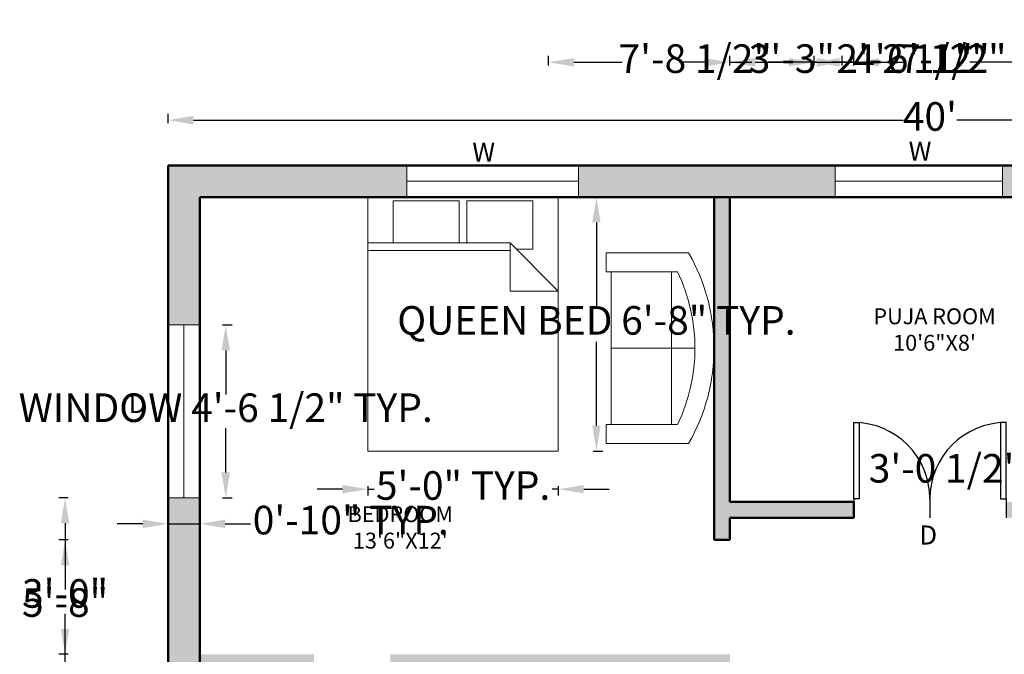
# Model space of a CAD drawing. Units: inches. Extents: x 2568 to 3190, y 746 to 1467.
# Tile 6 of 7: x 2588 to 2898, y 1267 to 1467. Entities that reach past the tile are written whole.
import ezdxf

# ---------------------------------------------------------------- set-up
doc = ezdxf.new("R2010")
doc.units = ezdxf.units.IN
for name, color, linetype, lineweight in [('A-ANNO-DIMS', 2, 'Continuous', 18), ('A-ANNO-TEXT', 7, 'Continuous', 18), ('A-AREA-IDEN', 7, 'Continuous', 25), ('A-DOOR', 3, 'Continuous', 25), ('A-FURN', 8, 'Continuous', 18), ('A-GLAZ', 4, 'Continuous', 20), ('A-WALL', 7, 'Continuous', 50), ('A-WALL-PATT', 252, 'Continuous', 13)]:
    doc.layers.add(name, color=color, linetype=linetype, lineweight=lineweight)
doc.styles.get("Standard").update_dxf_attribs({"font": 'arial.ttf'})
doc.dimstyles.new('ISO-25', dxfattribs={"dimtxt": 9, "dimasz": 8, "dimexe": 2, "dimexo": 1, "dimtad": 0, "dimtih": 1, "dimtoh": 1, "dimdec": 1, "dimlunit": 3, "dimtxsty": 'Standard', "dimcen": 2.5, "dimclrd": 1, "dimclre": 3, "dimclrt": 6, "dimadec": 0, "dimazin": 0, "dimtfac": 1, "dimtdec": 1, "dimtmove": 0, "dimatfit": 3, "dimfxl": 1, "dimfxlon": 1, "dimarcsym": 0})

# ---------------------------------------------------------------- blocks, each defined once
blk = doc.blocks.new('*U2')
for p, q in [((-24, 0), (-24, -6)), ((0, 0), (0, -6))]:
    blk.add_line(p, q)
blk.add_lwpolyline([(0, 0), (0, 24), (-1.75, 24), (-1.75, 0)], close=True)
blk.add_arc((0, 0), 24, 90, 180)
blk = doc.blocks.new('*U3')
for p, q in [((0, 0), (0, -6)), ((24, 0), (24, -6))]:
    blk.add_line(p, q)
blk.add_lwpolyline([(0, 0), (0, 24), (1.75, 24), (1.75, 0)], close=True)
blk.add_arc((0, 0), 24, 0, 90)
blk = doc.blocks.new('Bed - Queen')
for p, q in [((0, -80.00003), (0, 0)), ((0, 0), (59.99999, 0)), ((59.99999, 0), (59.99999, -80.00003)), ((7.99999, -1.2), (28.79998, -1.2)), ((7.99999, -14.4), (7.99999, -1.2)), ((28.79998, -1.2), (28.79998, -14.4)), ((31.19999, -1.2), (51.99999, -1.2)), ((31.19999, -14.4), (31.19999, -1.2)), ((51.99999, -1.2), (51.99999, -16.4)), ((0, -14.4), (44.8, -14.4)), ((59.99999, -29.6), (44.8, -14.4)), ((44.8, -14.4), (44.8, -29.6)), ((44.8, -16.8), (0, -16.8)), ((51.99999, -16.4), (46.79936, -16.4)), ((44.8, -29.6), (59.99999, -29.6)), ((59.99999, -80.00003), (0, -80.00003))]:
    blk.add_line(p, q)
blk = doc.blocks.new('*D13')
at = {"layer": 'A-ANNO-DIMS', "color": 0, "lineweight": -2, "transparency": 16777216}
for p, q in [((2634.52, 1434.58), (2634.52, 1437.58)), ((3114.52, 1434.58), (3114.52, 1437.58)), ((2642.52, 1435.58), (2866.08, 1435.58)), ((3106.52, 1435.58), (2882.97, 1435.58))]:
    blk.add_line(p, q, dxfattribs=at)
at = {"layer": 'A-ANNO-DIMS', "color": 0, "transparency": 16777216}
for points in [[(2642.52, 1436.91), (2642.52, 1434.24), (2634.52, 1435.58)], [(3106.52, 1436.91), (3106.52, 1434.24), (3114.52, 1435.58)]]:
    blk.add_solid(points, dxfattribs=at)
at = {"layer": 'Defpoints', "color": 0, "transparency": 16777216}
for p in [(2634.52, 1435.58), (2634.52, 1421.35), (3114.52, 1421.35)]:
    blk.add_point(p, dxfattribs=at)
at = {"layer": 'A-ANNO-DIMS', "color": 0, "transparency": 16777216, "insert": (2874.52, 1435.58), "char_height": 9, "attachment_point": 5}
blk.add_mtext("40'", dxfattribs=at)
blk = doc.blocks.new('Sofa - Roundback Loveseat 5 ft.')
for p, q in [((0, -32.44198), (0, -5.99998)), ((-24, -33.99998), (-24, -11.46958)), ((24.00004, -33.99998), (24.00004, -11.46958)), ((-23.9998, -13.38178), (23.99986, -13.38178)), ((-24, -32.44198), (24.00004, -32.44198))]:
    blk.add_line(p, q)
for points in [[(-24, -33.99998), (-30, -33.99998), (-30, -7.99998)], [(30.00004, -7.99998), (30.00004, -33.99998), (24.00004, -33.99998)]]:
    blk.add_lwpolyline(points)
for centre, radius, start, end in [((0, -60.24998), 60.24998, 60.13715, 119.8628), ((0, -61.38438), 55.38444, 64.32083, 115.6792)]:
    blk.add_arc(centre, radius, start, end)
blk = doc.blocks.new('WIN-BED-UPPER-54.46')
for p, q in [((5, 54.46), (-5, 54.46)), ((0, 54.46), (0, 0)), ((5, 0), (-5, 0))]:
    blk.add_line(p, q)
blk = doc.blocks.new('*D21')
at = {"layer": 'A-ANNO-DIMS', "color": 3, "lineweight": -2, "transparency": 16777216}
for p, q in [((2768.47, 1411.35), (2771.47, 1411.35)), ((2768.47, 1331.35), (2771.47, 1331.35))]:
    blk.add_line(p, q, dxfattribs=at)
at = {"layer": 'A-ANNO-DIMS', "color": 1, "lineweight": -2, "transparency": 16777216}
for p, q in [((2769.47, 1403.35), (2769.47, 1376.9)), ((2769.47, 1339.35), (2769.47, 1365.79))]:
    blk.add_line(p, q, dxfattribs=at)
at = {"layer": 'A-ANNO-DIMS', "color": 1, "transparency": 16777216}
for points in [[(2768.14, 1403.35), (2770.8, 1403.35), (2769.47, 1411.35)], [(2768.14, 1339.35), (2770.8, 1339.35), (2769.47, 1331.35)]]:
    blk.add_solid(points, dxfattribs=at)
at = {"layer": 'Defpoints', "color": 0, "transparency": 16777216}
for p in [(2757.47, 1411.35), (2769.47, 1411.35), (2757.47, 1331.35)]:
    blk.add_point(p, dxfattribs=at)
at = {"layer": 'A-ANNO-DIMS', "color": 6, "transparency": 16777216, "insert": (2769.47, 1371.35), "char_height": 9, "attachment_point": 5}
blk.add_mtext('QUEEN BED 6\'-8" TYP.', dxfattribs=at)
blk = doc.blocks.new('*D22')
at = {"layer": 'A-ANNO-DIMS', "color": 1, "lineweight": -2, "transparency": 16777216}
for p, q in [((2689.47, 1319.35), (2681.47, 1319.35)), ((2697.47, 1319.35), (2699.42, 1319.35)), ((2757.47, 1319.35), (2755.53, 1319.35)), ((2765.47, 1319.35), (2773.47, 1319.35))]:
    blk.add_line(p, q, dxfattribs=at)
at = {"layer": 'A-ANNO-DIMS', "color": 3, "lineweight": -2, "transparency": 16777216}
for p, q in [((2697.47, 1320.35), (2697.47, 1317.35)), ((2757.47, 1320.35), (2757.47, 1317.35))]:
    blk.add_line(p, q, dxfattribs=at)
at = {"layer": 'A-ANNO-DIMS', "color": 1, "transparency": 16777216}
for points in [[(2689.47, 1320.68), (2689.47, 1318.02), (2697.47, 1319.35)], [(2765.47, 1320.68), (2765.47, 1318.02), (2757.47, 1319.35)]]:
    blk.add_solid(points, dxfattribs=at)
at = {"layer": 'Defpoints', "color": 0, "transparency": 16777216}
for p in [(2697.47, 1331.35), (2757.47, 1331.35), (2757.47, 1319.35)]:
    blk.add_point(p, dxfattribs=at)
at = {"layer": 'A-ANNO-DIMS', "color": 6, "transparency": 16777216, "insert": (2727.47, 1319.35), "char_height": 9, "attachment_point": 5}
blk.add_mtext('5\'-0" TYP.', dxfattribs=at)
blk = doc.blocks.new('*D24')
at = {"layer": 'A-ANNO-DIMS', "color": 1, "lineweight": -2, "transparency": 16777216}
for p, q in [((2939.86, 1324.76), (2931.86, 1324.76)), ((2968.52, 1324.76), (2947.86, 1324.76))]:
    blk.add_line(p, q, dxfattribs=at)
at = {"layer": 'A-ANNO-DIMS', "color": 3, "lineweight": -2, "transparency": 16777216}
for p, q in [((2939.86, 1325.76), (2939.86, 1322.76)), ((2976.52, 1325.76), (2976.52, 1322.76))]:
    blk.add_line(p, q, dxfattribs=at)
at = {"layer": 'A-ANNO-DIMS', "color": 1, "transparency": 16777216}
for points in [[(2947.86, 1326.09), (2947.86, 1323.43), (2939.86, 1324.76)], [(2968.52, 1326.09), (2968.52, 1323.43), (2976.52, 1324.76)]]:
    blk.add_solid(points, dxfattribs=at)
at = {"layer": 'Defpoints', "color": 0, "transparency": 16777216}
for p in [(2939.86, 1333.76), (2976.52, 1333.76), (2939.86, 1324.76)]:
    blk.add_point(p, dxfattribs=at)
at = {"layer": 'A-ANNO-DIMS', "color": 6, "transparency": 16777216, "insert": (2893.32, 1324.76), "char_height": 9, "attachment_point": 5}
blk.add_mtext('3\'-0 1/2" TYP.', dxfattribs=at)
blk = doc.blocks.new('*D29')
at = {"layer": 'A-ANNO-DIMS', "color": 3, "lineweight": -2, "transparency": 16777216}
for p, q in [((2651.69, 1371.08), (2654.69, 1371.08)), ((2651.69, 1316.62), (2654.69, 1316.62))]:
    blk.add_line(p, q, dxfattribs=at)
at = {"layer": 'A-ANNO-DIMS', "color": 1, "lineweight": -2, "transparency": 16777216}
for p, q in [((2652.69, 1363.08), (2652.69, 1349.13)), ((2652.69, 1324.62), (2652.69, 1338.56))]:
    blk.add_line(p, q, dxfattribs=at)
at = {"layer": 'A-ANNO-DIMS', "color": 1, "transparency": 16777216}
for points in [[(2651.36, 1363.08), (2654.02, 1363.08), (2652.69, 1371.08)], [(2651.36, 1324.62), (2654.02, 1324.62), (2652.69, 1316.62)]]:
    blk.add_solid(points, dxfattribs=at)
at = {"layer": 'Defpoints', "color": 0, "transparency": 16777216}
for p in [(2644.52, 1371.08), (2652.69, 1371.08), (2644.52, 1316.62)]:
    blk.add_point(p, dxfattribs=at)
at = {"layer": 'A-ANNO-DIMS', "color": 6, "transparency": 16777216, "insert": (2652.69, 1343.85), "char_height": 9, "attachment_point": 5}
blk.add_mtext('WINDOW 4\'-6 1/2" TYP.', dxfattribs=at)
blk = doc.blocks.new('*D30')
at = {"layer": 'A-ANNO-DIMS', "color": 3, "lineweight": -2, "transparency": 16777216}
for p, q in [((2634.52, 1309.45), (2634.52, 1306.45)), ((2644.52, 1309.45), (2644.52, 1306.45))]:
    blk.add_line(p, q, dxfattribs=at)
at = {"layer": 'A-ANNO-DIMS', "color": 1, "lineweight": -2, "transparency": 16777216}
for p, q in [((2626.52, 1308.45), (2618.52, 1308.45)), ((2634.52, 1308.45), (2644.52, 1308.45)), ((2652.52, 1308.45), (2660.52, 1308.45))]:
    blk.add_line(p, q, dxfattribs=at)
at = {"layer": 'A-ANNO-DIMS', "color": 1, "transparency": 16777216}
for points in [[(2626.52, 1309.78), (2626.52, 1307.11), (2634.52, 1308.45)], [(2652.52, 1309.78), (2652.52, 1307.11), (2644.52, 1308.45)]]:
    blk.add_solid(points, dxfattribs=at)
at = {"layer": 'Defpoints', "color": 0, "transparency": 16777216}
for p in [(2634.52, 1316.62), (2644.52, 1316.62), (2644.52, 1308.45)]:
    blk.add_point(p, dxfattribs=at)
at = {"layer": 'A-ANNO-DIMS', "color": 6, "transparency": 16777216, "insert": (2692.07, 1308.45), "char_height": 9, "attachment_point": 5}
blk.add_mtext('0\'-10" TYP.', dxfattribs=at)
blk = doc.blocks.new('*D31')
at = {"layer": 'A-ANNO-DIMS', "color": 1, "lineweight": -2, "transparency": 16777216}
for p, q in [((2648.47, 1248.37), (2648.47, 1256.37)), ((2648.47, 1256.37), (2656.47, 1256.37)), ((2648.47, 1230.08), (2648.47, 1240.37))]:
    blk.add_line(p, q, dxfattribs=at)
at = {"layer": 'A-ANNO-DIMS', "color": 3, "lineweight": -2, "transparency": 16777216}
for p, q in [((2647.47, 1248.37), (2650.47, 1248.37)), ((2647.47, 1222.08), (2650.47, 1222.08))]:
    blk.add_line(p, q, dxfattribs=at)
at = {"layer": 'A-ANNO-DIMS', "color": 1, "transparency": 16777216}
for points in [[(2647.13, 1240.37), (2649.8, 1240.37), (2648.47, 1248.37)], [(2647.13, 1230.08), (2649.8, 1230.08), (2648.47, 1222.08)]]:
    blk.add_solid(points, dxfattribs=at)
at = {"layer": 'Defpoints', "color": 0, "transparency": 16777216}
for p in [(2644.52, 1248.37), (2648.47, 1248.37), (2644.52, 1222.08)]:
    blk.add_point(p, dxfattribs=at)
at = {"layer": 'A-ANNO-DIMS', "color": 6, "transparency": 16777216, "insert": (2724.52, 1256.37), "char_height": 9, "attachment_point": 5}
blk.add_mtext('WINDOW 2\'-2 1/2" TYP.', dxfattribs=at)
blk = doc.blocks.new('*D39')
at = {"layer": 'A-ANNO-DIMS', "color": 3, "lineweight": -2, "transparency": 16777216}
for p, q in [((2644.52, 760.85), (2644.52, 757.85)), ((2709.74, 760.85), (2709.74, 757.85))]:
    blk.add_line(p, q, dxfattribs=at)
at = {"layer": 'A-ANNO-DIMS', "color": 1, "lineweight": -2, "transparency": 16777216}
for p, q in [((2652.52, 759.85), (2664.54, 759.85)), ((2701.74, 759.85), (2689.72, 759.85))]:
    blk.add_line(p, q, dxfattribs=at)
at = {"layer": 'A-ANNO-DIMS', "color": 1, "transparency": 16777216}
for points in [[(2652.52, 761.18), (2652.52, 758.51), (2644.52, 759.85)], [(2701.74, 761.18), (2701.74, 758.51), (2709.74, 759.85)]]:
    blk.add_solid(points, dxfattribs=at)
at = {"layer": 'Defpoints', "color": 0, "transparency": 16777216}
for p in [(2644.52, 1411.35), (2709.74, 1411.35), (2709.74, 759.85)]:
    blk.add_point(p, dxfattribs=at)
at = {"layer": 'A-ANNO-DIMS', "color": 6, "transparency": 16777216, "insert": (2677.13, 759.85), "char_height": 9, "attachment_point": 5}
blk.add_mtext('5\'-5"', dxfattribs=at)
blk = doc.blocks.new('*D40')
at = {"layer": 'A-ANNO-DIMS', "color": 3, "lineweight": -2, "transparency": 16777216}
for p, q in [((2709.74, 760.85), (2709.74, 757.85)), ((2763.78, 760.85), (2763.78, 757.85))]:
    blk.add_line(p, q, dxfattribs=at)
at = {"layer": 'A-ANNO-DIMS', "color": 1, "lineweight": -2, "transparency": 16777216}
for p, q in [((2717.74, 759.85), (2723.99, 759.85)), ((2755.78, 759.85), (2749.52, 759.85))]:
    blk.add_line(p, q, dxfattribs=at)
at = {"layer": 'A-ANNO-DIMS', "color": 1, "transparency": 16777216}
for points in [[(2717.74, 761.18), (2717.74, 758.51), (2709.74, 759.85)], [(2755.78, 761.18), (2755.78, 758.51), (2763.78, 759.85)]]:
    blk.add_solid(points, dxfattribs=at)
at = {"layer": 'Defpoints', "color": 0, "transparency": 16777216}
for p in [(2709.74, 1411.35), (2763.78, 1411.35), (2763.78, 759.85)]:
    blk.add_point(p, dxfattribs=at)
at = {"layer": 'A-ANNO-DIMS', "color": 6, "transparency": 16777216, "insert": (2736.76, 759.85), "char_height": 9, "attachment_point": 5}
blk.add_mtext('4\'-6"', dxfattribs=at)
blk = doc.blocks.new('*D41')
at = {"layer": 'A-ANNO-DIMS', "color": 3, "lineweight": -2, "transparency": 16777216}
for p, q in [((2811.52, 760.85), (2811.52, 757.85)), ((2844.66, 760.85), (2844.66, 757.85))]:
    blk.add_line(p, q, dxfattribs=at)
at = {"layer": 'A-ANNO-DIMS', "color": 1, "lineweight": -2, "transparency": 16777216}
for p, q in [((2803.52, 759.85), (2795.52, 759.85)), ((2811.52, 759.85), (2815.43, 759.85)), ((2844.66, 759.85), (2840.76, 759.85)), ((2852.66, 759.85), (2860.66, 759.85))]:
    blk.add_line(p, q, dxfattribs=at)
at = {"layer": 'A-ANNO-DIMS', "color": 1, "transparency": 16777216}
for points in [[(2803.52, 761.18), (2803.52, 758.51), (2811.52, 759.85)], [(2852.66, 761.18), (2852.66, 758.51), (2844.66, 759.85)]]:
    blk.add_solid(points, dxfattribs=at)
at = {"layer": 'Defpoints', "color": 0, "transparency": 16777216}
for p in [(2811.52, 1411.35), (2844.66, 1411.35), (2844.66, 759.85)]:
    blk.add_point(p, dxfattribs=at)
at = {"layer": 'A-ANNO-DIMS', "color": 6, "transparency": 16777216, "insert": (2828.09, 759.85), "char_height": 9, "attachment_point": 5}
blk.add_mtext('2\'-9"', dxfattribs=at)
blk = doc.blocks.new('*D42')
at = {"layer": 'A-ANNO-DIMS', "color": 3, "lineweight": -2, "transparency": 16777216}
for p, q in [((2844.66, 760.85), (2844.66, 757.85)), ((2897.43, 760.85), (2897.43, 757.85))]:
    blk.add_line(p, q, dxfattribs=at)
at = {"layer": 'A-ANNO-DIMS', "color": 1, "lineweight": -2, "transparency": 16777216}
for p, q in [((2852.66, 759.85), (2858.28, 759.85)), ((2889.43, 759.85), (2883.81, 759.85))]:
    blk.add_line(p, q, dxfattribs=at)
at = {"layer": 'A-ANNO-DIMS', "color": 1, "transparency": 16777216}
for points in [[(2852.66, 761.18), (2852.66, 758.51), (2844.66, 759.85)], [(2889.43, 761.18), (2889.43, 758.51), (2897.43, 759.85)]]:
    blk.add_solid(points, dxfattribs=at)
at = {"layer": 'Defpoints', "color": 0, "transparency": 16777216}
for p in [(2844.66, 1411.35), (2897.43, 1411.35), (2897.43, 759.85)]:
    blk.add_point(p, dxfattribs=at)
at = {"layer": 'A-ANNO-DIMS', "color": 6, "transparency": 16777216, "insert": (2871.04, 759.85), "char_height": 9, "attachment_point": 5}
blk.add_mtext('4\'-5"', dxfattribs=at)
blk = doc.blocks.new('*D47')
at = {"layer": 'A-ANNO-DIMS', "color": 3, "lineweight": -2, "transparency": 16777216}
for p, q in [((2754.37, 1452.8), (2754.37, 1455.8)), ((2846.86, 1452.8), (2846.86, 1455.8))]:
    blk.add_line(p, q, dxfattribs=at)
at = {"layer": 'A-ANNO-DIMS', "color": 1, "lineweight": -2, "transparency": 16777216}
for p, q in [((2762.37, 1453.8), (2777.58, 1453.8)), ((2838.86, 1453.8), (2823.65, 1453.8))]:
    blk.add_line(p, q, dxfattribs=at)
at = {"layer": 'A-ANNO-DIMS', "color": 1, "transparency": 16777216}
for points in [[(2762.37, 1455.13), (2762.37, 1452.47), (2754.37, 1453.8)], [(2838.86, 1455.13), (2838.86, 1452.47), (2846.86, 1453.8)]]:
    blk.add_solid(points, dxfattribs=at)
at = {"layer": 'Defpoints', "color": 0, "transparency": 16777216}
for p in [(2846.86, 1453.8), (2754.37, 831.35), (2846.86, 831.35)]:
    blk.add_point(p, dxfattribs=at)
at = {"layer": 'A-ANNO-DIMS', "color": 6, "transparency": 16777216, "insert": (2800.61, 1453.8), "char_height": 9, "attachment_point": 5}
blk.add_mtext('7\'-8 1/2"', dxfattribs=at)
blk = doc.blocks.new('*D50')
at = {"layer": 'A-ANNO-DIMS', "color": 3, "lineweight": -2, "transparency": 16777216}
for p, q in [((2846.86, 1452.8), (2846.86, 1455.8)), ((2902.21, 1452.8), (2902.21, 1455.8))]:
    blk.add_line(p, q, dxfattribs=at)
at = {"layer": 'A-ANNO-DIMS', "color": 1, "lineweight": -2, "transparency": 16777216}
for p, q in [((2838.86, 1453.8), (2830.86, 1453.8)), ((2846.86, 1453.8), (2851.29, 1453.8)), ((2902.21, 1453.8), (2897.79, 1453.8)), ((2910.21, 1453.8), (2918.21, 1453.8))]:
    blk.add_line(p, q, dxfattribs=at)
at = {"layer": 'A-ANNO-DIMS', "color": 1, "transparency": 16777216}
for points in [[(2838.86, 1455.13), (2838.86, 1452.47), (2846.86, 1453.8)], [(2910.21, 1455.13), (2910.21, 1452.47), (2902.21, 1453.8)]]:
    blk.add_solid(points, dxfattribs=at)
at = {"layer": 'Defpoints', "color": 0, "transparency": 16777216}
for p in [(2902.21, 1453.8), (2846.86, 831.35), (2902.21, 831.35)]:
    blk.add_point(p, dxfattribs=at)
at = {"layer": 'A-ANNO-DIMS', "color": 6, "transparency": 16777216, "insert": (2874.54, 1453.8), "char_height": 9, "attachment_point": 5}
blk.add_mtext('4\'-7 1/2"', dxfattribs=at)
blk = doc.blocks.new('*D53')
at = {"layer": 'A-ANNO-DIMS', "color": 1, "lineweight": -2, "transparency": 16777216}
for p, q in [((3146.97, 1323.35), (3146.97, 1331.35)), ((3146.97, 1331.35), (3154.97, 1331.35)), ((3146.97, 1310.35), (3146.97, 1315.35)), ((3146.97, 1302.35), (3146.97, 1294.35))]:
    blk.add_line(p, q, dxfattribs=at)
at = {"layer": 'A-ANNO-DIMS', "color": 3, "lineweight": -2, "transparency": 16777216}
for p, q in [((3145.97, 1315.35), (3148.97, 1315.35)), ((3145.97, 1310.35), (3148.97, 1310.35))]:
    blk.add_line(p, q, dxfattribs=at)
at = {"layer": 'A-ANNO-DIMS', "color": 1, "transparency": 16777216}
for points in [[(3145.64, 1323.35), (3148.31, 1323.35), (3146.97, 1315.35)], [(3145.64, 1302.35), (3148.31, 1302.35), (3146.97, 1310.35)]]:
    blk.add_solid(points, dxfattribs=at)
at = {"layer": 'Defpoints', "color": 0, "transparency": 16777216}
for p in [(2811.52, 1315.35), (3146.97, 1315.35), (2811.52, 1310.35)]:
    blk.add_point(p, dxfattribs=at)
at = {"layer": 'A-ANNO-DIMS', "color": 6, "transparency": 16777216, "insert": (3167.56, 1331.35), "char_height": 9, "attachment_point": 5}
blk.add_mtext('0\'-5"', dxfattribs=at)
blk = doc.blocks.new('*D54')
at = {"layer": 'A-ANNO-DIMS', "color": 3, "lineweight": -2, "transparency": 16777216}
for p, q in [((2850.52, 760.85), (2850.52, 757.85)), ((2898.52, 760.85), (2898.52, 757.85))]:
    blk.add_line(p, q, dxfattribs=at)
at = {"layer": 'A-ANNO-DIMS', "color": 1, "lineweight": -2, "transparency": 16777216}
for p, q in [((2858.52, 759.85), (2861.75, 759.85)), ((2890.52, 759.85), (2887.29, 759.85))]:
    blk.add_line(p, q, dxfattribs=at)
at = {"layer": 'A-ANNO-DIMS', "color": 1, "transparency": 16777216}
for points in [[(2858.52, 761.18), (2858.52, 758.51), (2850.52, 759.85)], [(2890.52, 761.18), (2890.52, 758.51), (2898.52, 759.85)]]:
    blk.add_solid(points, dxfattribs=at)
at = {"layer": 'Defpoints', "color": 0, "transparency": 16777216}
for p in [(2850.52, 1310.35), (2898.52, 1310.35), (2898.52, 759.85)]:
    blk.add_point(p, dxfattribs=at)
at = {"layer": 'A-ANNO-DIMS', "color": 6, "transparency": 16777216, "insert": (2874.52, 759.85), "char_height": 9, "attachment_point": 5}
blk.add_mtext('4\'-0"', dxfattribs=at)
blk = doc.blocks.new('*D55')
at = {"layer": 'A-ANNO-DIMS', "color": 3, "lineweight": -2, "transparency": 16777216}
for p, q in [((2603.07, 1303.35), (2600.07, 1303.35)), ((2603.07, 1267.35), (2600.07, 1267.35))]:
    blk.add_line(p, q, dxfattribs=at)
at = {"layer": 'A-ANNO-DIMS', "color": 1, "lineweight": -2, "transparency": 16777216}
for p, q in [((2602.07, 1295.35), (2602.07, 1290.57)), ((2602.07, 1275.35), (2602.07, 1280.13))]:
    blk.add_line(p, q, dxfattribs=at)
at = {"layer": 'A-ANNO-DIMS', "color": 1, "transparency": 16777216}
for points in [[(2600.74, 1295.35), (2603.41, 1295.35), (2602.07, 1303.35)], [(2600.74, 1275.35), (2603.41, 1275.35), (2602.07, 1267.35)]]:
    blk.add_solid(points, dxfattribs=at)
at = {"layer": 'Defpoints', "color": 0, "transparency": 16777216}
for p in [(2942.52, 1303.35), (2602.07, 1267.35), (2941.77, 1267.35)]:
    blk.add_point(p, dxfattribs=at)
at = {"layer": 'A-ANNO-DIMS', "color": 6, "transparency": 16777216, "insert": (2602.07, 1285.35), "char_height": 9, "attachment_point": 5}
blk.add_mtext('3\'-0"', dxfattribs=at)
blk = doc.blocks.new('*D71')
at = {"layer": 'A-ANNO-DIMS', "color": 3, "lineweight": -2, "transparency": 16777216}
for p, q in [((2603.07, 1316.62), (2600.07, 1316.62)), ((2603.07, 1248.37), (2600.07, 1248.37))]:
    blk.add_line(p, q, dxfattribs=at)
at = {"layer": 'A-ANNO-DIMS', "color": 1, "lineweight": -2, "transparency": 16777216}
for p, q in [((2602.07, 1308.62), (2602.07, 1287.71)), ((2602.07, 1256.37), (2602.07, 1277.27))]:
    blk.add_line(p, q, dxfattribs=at)
at = {"layer": 'A-ANNO-DIMS', "color": 1, "transparency": 16777216}
for points in [[(2600.74, 1308.62), (2603.41, 1308.62), (2602.07, 1316.62)], [(2600.74, 1256.37), (2603.41, 1256.37), (2602.07, 1248.37)]]:
    blk.add_solid(points, dxfattribs=at)
at = {"layer": 'Defpoints', "color": 0, "transparency": 16777216}
for p in [(2602.07, 1316.62), (2634.52, 1316.62), (2634.52, 1248.37)]:
    blk.add_point(p, dxfattribs=at)
at = {"layer": 'A-ANNO-DIMS', "color": 6, "transparency": 16777216, "insert": (2602.07, 1282.49), "char_height": 9, "attachment_point": 5}
blk.add_mtext('5\'-8"', dxfattribs=at)
blk = doc.blocks.new('*D80')
at = {"layer": 'A-ANNO-DIMS', "color": 3, "lineweight": -2, "transparency": 16777216}
for p, q in [((2838.1, 1452.8), (2838.1, 1455.8)), ((2910.92, 1452.8), (2910.92, 1455.8))]:
    blk.add_line(p, q, dxfattribs=at)
at = {"layer": 'A-ANNO-DIMS', "color": 1, "lineweight": -2, "transparency": 16777216}
for p, q in [((2846.1, 1453.8), (2861.9, 1453.8)), ((2902.92, 1453.8), (2887.12, 1453.8))]:
    blk.add_line(p, q, dxfattribs=at)
at = {"layer": 'A-ANNO-DIMS', "color": 1, "transparency": 16777216}
for points in [[(2846.1, 1455.13), (2846.1, 1452.47), (2838.1, 1453.8)], [(2902.92, 1455.13), (2902.92, 1452.47), (2910.92, 1453.8)]]:
    blk.add_solid(points, dxfattribs=at)
at = {"layer": 'Defpoints', "color": 0, "transparency": 16777216}
for p in [(2910.92, 1453.8), (2838.1, 1075.35), (2910.92, 1075.35)]:
    blk.add_point(p, dxfattribs=at)
at = {"layer": 'A-ANNO-DIMS', "color": 6, "transparency": 16777216, "insert": (2874.51, 1453.8), "char_height": 9, "attachment_point": 5}
blk.add_mtext('6\'-1"', dxfattribs=at)
blk = doc.blocks.new('*D81')
at = {"layer": 'A-ANNO-DIMS', "color": 3, "lineweight": -2, "transparency": 16777216}
for p, q in [((2811.52, 1452.8), (2811.52, 1455.8)), ((2838.1, 1452.8), (2838.1, 1455.8))]:
    blk.add_line(p, q, dxfattribs=at)
at = {"layer": 'A-ANNO-DIMS', "color": 1, "lineweight": -2, "transparency": 16777216}
for p, q in [((2819.52, 1453.8), (2830.1, 1453.8)), ((2838.1, 1453.8), (2846.1, 1453.8))]:
    blk.add_line(p, q, dxfattribs=at)
at = {"layer": 'A-ANNO-DIMS', "color": 1, "transparency": 16777216}
for points in [[(2819.52, 1455.13), (2819.52, 1452.47), (2811.52, 1453.8)], [(2830.1, 1455.13), (2830.1, 1452.47), (2838.1, 1453.8)]]:
    blk.add_solid(points, dxfattribs=at)
at = {"layer": 'Defpoints', "color": 0, "transparency": 16777216}
for p in [(2838.1, 1453.8), (2811.52, 1075.35), (2838.1, 1075.35)]:
    blk.add_point(p, dxfattribs=at)
at = {"layer": 'A-ANNO-DIMS', "color": 6, "transparency": 16777216, "insert": (2869.24, 1453.8), "char_height": 9, "attachment_point": 5}
blk.add_mtext('2\'-2 1/2"', dxfattribs=at)
blk = doc.blocks.new('*D82')
at = {"layer": 'A-ANNO-DIMS', "color": 3, "lineweight": -2, "transparency": 16777216}
for p, q in [((2811.52, 1452.8), (2811.52, 1455.8)), ((2850.52, 1452.8), (2850.52, 1455.8))]:
    blk.add_line(p, q, dxfattribs=at)
at = {"layer": 'A-ANNO-DIMS', "color": 1, "lineweight": -2, "transparency": 16777216}
for p, q in [((2803.52, 1453.8), (2795.52, 1453.8)), ((2811.52, 1453.8), (2818.44, 1453.8)), ((2850.52, 1453.8), (2843.61, 1453.8)), ((2858.52, 1453.8), (2866.52, 1453.8))]:
    blk.add_line(p, q, dxfattribs=at)
at = {"layer": 'A-ANNO-DIMS', "color": 1, "transparency": 16777216}
for points in [[(2803.52, 1455.13), (2803.52, 1452.47), (2811.52, 1453.8)], [(2858.52, 1455.13), (2858.52, 1452.47), (2850.52, 1453.8)]]:
    blk.add_solid(points, dxfattribs=at)
at = {"layer": 'Defpoints', "color": 0, "transparency": 16777216}
for p in [(2811.52, 1453.8), (2811.52, 1315.35), (2850.52, 1315.35)]:
    blk.add_point(p, dxfattribs=at)
at = {"layer": 'A-ANNO-DIMS', "color": 6, "transparency": 16777216, "insert": (2831.02, 1453.8), "char_height": 9, "attachment_point": 5}
blk.add_mtext('3\'-3"', dxfattribs=at)

msp = doc.modelspace()

# ---------------------------------------------------------------- hatches: boundary and pattern name
at = {"layer": 'A-WALL-PATT'}
h = msp.add_hatch(color=256, dxfattribs=at)
h.dxf.hatch_style = 1
h.paths.add_polyline_path([(2709.74, 1411.35), (2709.74, 1421.35), (2634.52, 1421.35), (2634.52, 1371.08), (2644.52, 1371.08), (2644.52, 1411.35)])
h.paths.add_polyline_path([(2844.66, 1411.35), (2844.66, 1421.35), (2763.78, 1421.35), (2763.78, 1411.35)])
h.paths.add_polyline_path([(2996.2, 1411.35), (2996.2, 1421.35), (2897.43, 1421.35), (2897.43, 1411.35)])
h.paths.add_polyline_path([(3104.52, 1411.35), (3104.52, 1371.08), (3114.52, 1371.08), (3114.52, 1421.35), (3052.64, 1421.35), (3052.64, 1411.35)])
h.paths.add_polyline_path([(3114.52, 1316.62), (3104.52, 1316.62), (3104.52, 1248.37), (3114.52, 1248.37)])
h.paths.add_polyline_path([(3104.52, 1174.04), (3114.52, 1174.04), (3114.52, 1222.08), (3104.52, 1222.08)])
h.paths.add_polyline_path([(3104.52, 1020.11), (3114.52, 1020.11), (3114.52, 1113), (3104.52, 1113)])
h.paths.add_polyline_path([(3104.52, 920.42), (3114.52, 920.42), (3114.52, 992.96), (3104.52, 992.96)])
h.paths.add_polyline_path([(3114.52, 821.35), (3114.52, 865.93), (3104.52, 865.93), (3104.52, 831.35), (3055.78, 831.35), (3055.78, 821.35)])
h.paths.add_polyline_path([(2902.21, 831.35), (2902.21, 821.35), (2986.63, 821.35), (2986.63, 831.35)])
h.paths.add_polyline_path([(2634.52, 821.35), (2676.76, 821.35), (2676.76, 831.35), (2644.52, 831.35), (2644.52, 865.93), (2634.52, 865.93)])
h.paths.add_polyline_path([(2754.37, 821.35), (2846.86, 821.35), (2846.86, 831.35), (2754.37, 831.35)])
h.paths.add_polyline_path([(2644.52, 920.42), (2644.52, 1002.57), (2634.52, 1002.57), (2634.52, 920.42)])
h.paths.add_polyline_path([(2644.52, 1044.16), (2644.52, 1113), (2634.52, 1113), (2634.52, 1044.16)])
h.paths.add_polyline_path([(2644.52, 1248.37), (2644.52, 1316.62), (2634.52, 1316.62), (2634.52, 1248.37)])
h.paths.add_polyline_path([(2634.52, 1222.08), (2634.52, 1174.04), (2644.52, 1174.04), (2644.52, 1222.08)])
h = msp.add_hatch(color=256, dxfattribs=at)
h.dxf.hatch_style = 1
h.paths.add_polyline_path([(2811.52, 1411.35), (2806.52, 1411.35), (2806.52, 1303.35), (2811.52, 1303.35), (2811.52, 1310.35), (2850.52, 1310.35), (2850.52, 1315.35), (2811.52, 1315.35)])
h.paths.add_polyline_path([(2942.52, 1411.35), (2937.52, 1411.35), (2937.52, 1315.35), (2898.52, 1315.35), (2898.52, 1310.35), (2937.52, 1310.35), (2937.52, 1303.35), (2942.52, 1303.35)])
h.paths.add_polyline_path([(2811.52, 1267.35), (2704.52, 1267.35), (2704.52, 1261.35), (2704.52, 1237.35), (2704.52, 1202.35), (2644.52, 1202.35), (2644.52, 1197.35), (2806.52, 1197.35), (2806.52, 1191.38), (2811.52, 1191.38), (2811.52, 1202.35), (2793.52, 1202.35), (2793.52, 1232.35), (2788.52, 1232.35), (2788.52, 1202.35), (2709.52, 1202.35), (2709.52, 1262.35), (2788.52, 1262.35), (2788.52, 1256.35), (2793.52, 1256.35), (2793.52, 1262.35), (2811.52, 1262.35)])
h.paths.add_polyline_path([(2680.52, 1267.35), (2644.52, 1267.35), (2644.52, 1261.35), (2680.52, 1261.35)])
h.paths.add_polyline_path([(3044.52, 1267.35), (2937.52, 1267.35), (2937.52, 1262.35), (2955.52, 1262.35), (2955.52, 1256.35), (2960.52, 1256.35), (2960.52, 1262.35), (3039.52, 1262.35), (3039.52, 1202.35), (2960.52, 1202.35), (2960.52, 1232.35), (2955.52, 1232.35), (2955.52, 1202.35), (2937.52, 1202.35), (2937.52, 1191.38), (2942.52, 1191.38), (2942.52, 1197.35), (3104.52, 1197.35), (3104.52, 1202.35), (3044.52, 1202.35)])
h.paths.add_polyline_path([(3104.52, 1267.35), (3072.52, 1267.35), (3072.52, 1262.35), (3104.52, 1262.35)])
h.paths.add_polyline_path([(2838.1, 1075.35), (2811.52, 1075.35), (2811.52, 1155.35), (2806.52, 1155.35), (2806.52, 1075.35), (2644.52, 1075.35), (2644.52, 1070.35), (2806.52, 1070.35), (2811.52, 1070.35), (2838.1, 1070.35)])
h.paths.add_polyline_path([(3104.52, 1075.35), (2942.52, 1075.35), (2942.52, 1155.38), (2937.52, 1155.38), (2937.52, 1075.35), (2910.92, 1075.35), (2910.92, 1070.35), (2937.52, 1070.35), (3104.52, 1070.35)])
h.paths.add_polyline_path([(2811.52, 1038.35), (2806.52, 1038.35), (2806.52, 980.35), (2644.52, 980.35), (2644.52, 975.35), (2806.52, 975.35), (2806.52, 969.37), (2811.52, 969.37), (2811.52, 975.35)])
h.paths.add_polyline_path([(3104.52, 980.35), (2937.52, 980.35), (2937.52, 969.35), (2942.52, 969.35), (2942.52, 975.35), (3104.52, 975.35)])
h.paths.add_polyline_path([(3104.52, 1034.35), (3039.52, 1034.35), (3039.52, 1004.35), (3044.52, 1004.35), (3044.52, 1029.35), (3104.52, 1029.35)])
h.paths.add_polyline_path([(2942.52, 933.35), (2937.52, 933.35), (2937.52, 831.35), (2942.52, 831.35)])
h.paths.add_polyline_path([(2811.52, 933.37), (2806.52, 933.37), (2806.52, 831.35), (2811.52, 831.35)])

# ---------------------------------------------------------------- linework, layer by layer
at = {"layer": 'A-GLAZ'}
for p, q in [((2709.74, 1421.35), (2709.74, 1411.35)), ((2763.78, 1411.35), (2763.78, 1421.35)), ((2844.66, 1411.35), (2844.66, 1421.35)), ((2897.43, 1421.35), (2897.43, 1411.35)), ((2709.74, 1416.35), (2763.78, 1416.35)), ((2844.66, 1416.35), (2897.43, 1416.35))]:
    msp.add_line(p, q, dxfattribs=at)
at = {"layer": 'A-WALL'}
for p, q in [((2634.52, 1421.35), (2634.52, 821.35)), ((3114.52, 1421.35), (2634.52, 1421.35)), ((2644.52, 1411.35), (2644.52, 831.35)), ((3104.52, 1411.35), (2644.52, 1411.35)), ((2806.52, 1411.35), (2806.52, 1303.35)), ((2811.52, 1411.35), (2811.52, 1315.35)), ((2811.52, 1315.35), (2850.52, 1315.35)), ((2850.52, 1315.35), (2850.52, 1310.35)), ((2811.52, 1310.35), (2850.52, 1310.35)), ((2811.52, 1310.35), (2811.52, 1303.35)), ((2811.52, 1303.35), (2806.52, 1303.35))]:
    msp.add_line(p, q, dxfattribs=at)

# ---------------------------------------------------------------- block references
at = {"layer": 'A-DOOR'}
for name, p in [('*U3', (2850.52, 1316.35)), ('*U2', (2898.52, 1316.35))]:
    msp.add_blockref(name, p, dxfattribs=at)
at = {"layer": 'A-FURN'}
msp.add_blockref('Bed - Queen', (2697.47, 1411.35), dxfattribs=at)
at = {"layer": 'A-FURN', "rotation": 270}
msp.add_blockref('Sofa - Roundback Loveseat 5 ft.', (2806.52, 1363.76), dxfattribs=at)
at = {"layer": 'A-GLAZ'}
msp.add_blockref('WIN-BED-UPPER-54.46', (2639.52, 1316.62), dxfattribs=at)

# ---------------------------------------------------------------- texts
at = {"layer": 'A-ANNO-TEXT', "char_height": 6, "attachment_point": 1}
for s, insert in [('W', (2730.36, 1428.54)), ('W', (2867.83, 1428.85)), ('D', (2622.08, 1349.34)), ('D', (2871.18, 1307.92))]:
    msp.add_mtext_dynamic_manual_height_columns(s, width=7.7602, gutter_width=12.5, heights=[0], dxfattribs=dict(at, insert=insert))
at = {"layer": 'A-AREA-IDEN', "char_height": 5, "attachment_point": 1}
for s, insert in [('\\pxqc;PUJA ROOM\\P10\'6"X8\'', (2841.06, 1376.3)), ('\\pxqc;BEDROOM\\P13\'6"X12\'', (2672.75, 1313.99))]:
    msp.add_mtext_dynamic_manual_height_columns(s, width=69.8646, gutter_width=12.5, heights=[0], dxfattribs=dict(at, insert=insert))

# ---------------------------------------------------------------- dimensions: what is measured, and where the dimension line sits
at = {"layer": 'A-ANNO-DIMS'}
for base, p1, p2, override, picture, middle in [((2846.86, 1453.8), (2754.37, 831.35), (2846.86, 831.35), {"dimdec": 1, "dimlfac": 1, "dimrnd": 0, "dimzin": 1, "dimdsep": 46, "dimlunit": 4, "dimfrac": 2}, '*D47', (2800.61, 1453.8)), ((2838.1, 1453.8), (2811.52, 1075.35), (2838.1, 1075.35), {"dimdec": 1, "dimlfac": 1, "dimrnd": 0, "dimzin": 1, "dimdsep": 46, "dimlunit": 4, "dimfrac": 2}, '*D81', (2869.24, 1453.8)), ((2902.2147, 1453.7989), (2846.8636, 831.3489), (2902.2147, 831.3489), {"dimdec": 1, "dimlfac": 1, "dimrnd": 0, "dimzin": 1, "dimdsep": 46, "dimlunit": 4, "dimfrac": 2}, '*D50', (2874.5391, 1453.7989)), ((2811.52, 1453.8), (2850.52, 1315.35), (2811.52, 1315.35), {"dimdec": 1, "dimlfac": 1, "dimrnd": 0, "dimzin": 1, "dimdsep": 46, "dimlunit": 4, "dimfrac": 2}, '*D82', (2831.02, 1453.8)), ((2910.92, 1453.8), (2838.1, 1075.35), (2910.92, 1075.35), {"dimdec": 1, "dimlfac": 1, "dimrnd": 0, "dimzin": 1, "dimdsep": 46, "dimlunit": 4, "dimfrac": 2}, '*D80', (2874.51, 1453.8)), ((2634.52, 1435.58), (3114.52, 1421.35), (2634.52, 1421.35), {"dimclrd": 0, "dimclre": 0, "dimclrt": 0}, '*D13', (2874.52, 1435.58)), ((2709.74, 759.85), (2644.52, 1411.35), (2709.74, 1411.35), {"dimdec": 1, "dimlfac": 1, "dimrnd": 0, "dimzin": 1, "dimdsep": 46, "dimlunit": 4, "dimfrac": 2}, '*D39', (2677.13, 759.85)), ((2763.78, 759.85), (2709.74, 1411.35), (2763.78, 1411.35), {"dimdec": 1, "dimlfac": 1, "dimrnd": 0, "dimzin": 1, "dimdsep": 46, "dimlunit": 4, "dimfrac": 2}, '*D40', (2736.76, 759.85)), ((2844.66, 759.85), (2811.52, 1411.35), (2844.66, 1411.35), {"dimdec": 1, "dimlfac": 1, "dimrnd": 0, "dimzin": 1, "dimdsep": 46, "dimlunit": 4, "dimfrac": 2}, '*D41', (2828.09, 759.85)), ((2897.43, 759.85), (2844.66, 1411.35), (2897.43, 1411.35), {"dimdec": 1, "dimlfac": 1, "dimrnd": 0, "dimzin": 1, "dimdsep": 46, "dimlunit": 4, "dimfrac": 2}, '*D42', (2871.04, 759.85)), ((2898.52, 759.85), (2850.52, 1310.35), (2898.52, 1310.35), {"dimdec": 1, "dimlfac": 1, "dimrnd": 0, "dimzin": 1, "dimdsep": 46, "dimlunit": 4, "dimfrac": 2}, '*D54', (2874.52, 759.85))]:
    dim = msp.add_linear_dim(base=base, p1=p1, p2=p2, dimstyle='ISO-25', override=override, dxfattribs=at)
    dim.commit()
    dim.dimension.update_dxf_attribs({"geometry": picture, "text_midpoint": middle})
for base, p1, p2, angle, text, picture, middle in [((2769.47, 1411.35), (2757.47, 1331.35), (2757.47, 1411.35), 90, 'QUEEN BED <> TYP.', '*D21', (2769.47, 1371.35)), ((2652.69, 1371.08), (2644.52, 1316.62), (2644.52, 1371.08), 90, 'WINDOW <> TYP.', '*D29', (2652.69, 1343.85)), ((2939.86, 1324.76), (2976.52, 1333.76), (2939.86, 1333.76), 180, '<> TYP.', '*D24', (2893.32, 1324.76)), ((2648.47, 1248.37), (2644.52, 1222.08), (2644.52, 1248.37), 90, 'WINDOW <> TYP.', '*D31', (2724.52, 1256.37))]:
    dim = msp.add_linear_dim(base=base, p1=p1, p2=p2, angle=angle, text=text, dimstyle='ISO-25', override={"dimdec": 1, "dimlfac": 1, "dimrnd": 0, "dimzin": 1, "dimdsep": 46, "dimlunit": 4, "dimfrac": 2}, dxfattribs=at)
    dim.commit()
    dim.dimension.update_dxf_attribs({"geometry": picture, "text_midpoint": middle})
for base, p1, p2, picture, middle in [((3146.97, 1315.35), (2811.52, 1310.35), (2811.52, 1315.35), '*D53', (3167.56, 1331.35)), ((2602.0725, 1316.6152), (2634.5225, 1248.3665), (2634.5225, 1316.6152), '*D71', (2602.0725, 1282.4908)), ((2602.07, 1267.35), (2942.52, 1303.35), (2941.77, 1267.35), '*D55', (2602.07, 1285.35))]:
    dim = msp.add_linear_dim(base=base, p1=p1, p2=p2, angle=90, dimstyle='ISO-25', override={"dimdec": 1, "dimlfac": 1, "dimrnd": 0, "dimzin": 1, "dimdsep": 46, "dimlunit": 4, "dimfrac": 2}, dxfattribs=at)
    dim.commit()
    dim.dimension.update_dxf_attribs({"geometry": picture, "text_midpoint": middle})
for base, p1, p2, picture, middle in [((2757.47, 1319.35), (2697.47, 1331.35), (2757.47, 1331.35), '*D22', (2727.47, 1319.35)), ((2644.52, 1308.45), (2634.52, 1316.62), (2644.52, 1316.62), '*D30', (2692.07, 1308.45))]:
    dim = msp.add_linear_dim(base=base, p1=p1, p2=p2, text='<> TYP.', dimstyle='ISO-25', override={"dimdec": 1, "dimlfac": 1, "dimrnd": 0, "dimzin": 1, "dimdsep": 46, "dimlunit": 4, "dimfrac": 2}, dxfattribs=at)
    dim.commit()
    dim.dimension.update_dxf_attribs({"geometry": picture, "text_midpoint": middle})

doc.saveas('drawing.dxf')
